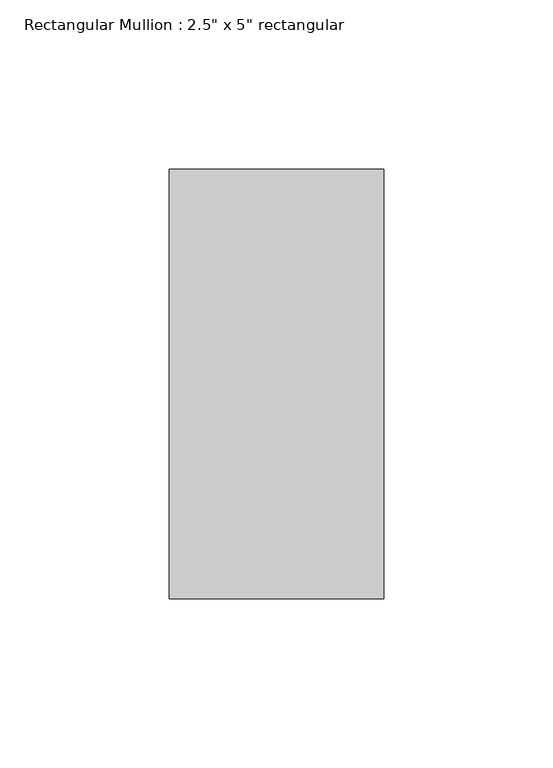
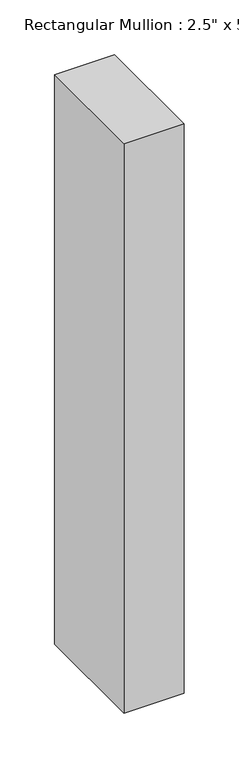
"""IFC4 building model written with IfcOpenShell, lengths in millimetres: member geometry."""

from ifc_helpers import new_model, si_unit, frame, origin, place, context, project, spatial, polyline, outline, extrude, source, transform, mapped, element, save


def member_5e365d0c(model_context):
    return source(origin(), model_context, "Body", "SweptSolid", [
        extrude(outline(polyline([(0.0, 63.5), (0.0, -63.5), (-63.5, -63.5), (-63.5, 63.5), (0.0, 63.5)])), frame((0.0, 0.0, -635.0), z_axis=(0.0, 0.0, 1.0), x_axis=(1.0, 0.0, 0.0)), (0.0, 0.0, 1.0), 635.0),
    ])


if __name__ == "__main__":
    model = new_model("IFC4")
    model_context = context("Model", 3, world=origin())
    ifc_project = project(units=[si_unit("LENGTHUNIT", "METRE", prefix="MILLI")], contexts=[model_context])
    site = spatial("IfcSite", under=ifc_project)
    building = spatial("IfcBuilding", under=site)
    placement = place(None, origin())
    member_shape = member_5e365d0c(model_context)
    element("IfcMember", 1, ObjectType="Rectangular Mullion : 2.5\" x 5\" rectangular", at=placement, inside=building, context=model_context, shape_type="MappedRepresentation", body=[
        mapped(member_shape, transform((0.0, 0.0, 0.0), x_axis=(1.0, 0.0, 0.0), y_axis=(0.0, 1.0, 0.0), z_axis=(0.0, 0.0, 1.0))),
    ])
    save(model, "model.ifc")

# Revit data of these elements
# Type "Rectangular Mullion : 2.5\" x 5\" rectangular"
#   built-in parameter 1007304 = 0.416667 (stored number, unit not read)
#   built-in parameter 1007301 = 0.104167 (stored number, unit not read)
#   built-in parameter 1007300 = 0.104167 (stored number, unit not read)
# Element 1 (IfcMember, "Rectangular Mullion : 2.5\" x 5\" rectangular")
#   Materials on its faces: "door colour"
# Materials
#   "door colour": class "Generic", colour RGB 120 120 120, transparency 0, Cost = 0
